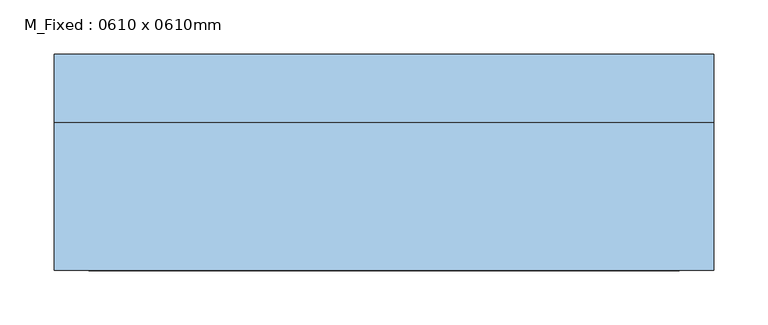
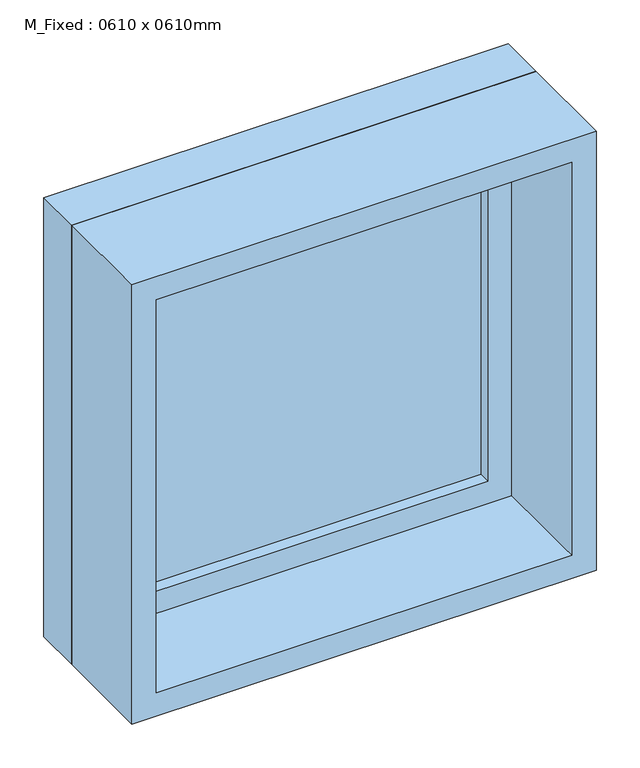
"""IFC4 building model written with IfcOpenShell, lengths in millimetres: window geometry, M_Fixed : 0610 x 0610mm."""

from ifc_helpers import new_model, si_unit, frame, origin, place, context, project, spatial, polyline, outline, extrude, source, transform, mapped, element, save


def m_fixed_0610_x_0610mm_cacddef9(model_context):
    return source(origin(), model_context, "Body", "SweptSolid", [
        extrude(outline(polyline([(-242.0, 78.0), (242.0, 78.0), (242.0, 66.0), (-242.0, 66.0), (-242.0, 78.0)])), frame((0.0, 0.0, 978.0), z_axis=(0.0, 0.0, 1.0), x_axis=(1.0, 0.0, 0.0)), (0.0, 0.0, 1.0), 484.0),
        extrude(outline(polyline([(1506.0, -286.0), (934.0, -286.0), (934.0, 286.0), (1506.0, 286.0), (1506.0, -286.0)]), holes=[polyline([(1462.0, -242.0), (1462.0, 242.0), (978.0, 242.0), (978.0, -242.0), (1462.0, -242.0)])]), frame((0.0, 50.0, 0.0), z_axis=(0.0, 1.0, 0.0), x_axis=(0.0, 0.0, 1.0)), (0.0, 0.0, 1.0), 44.0),
        extrude(outline(polyline([(1525.0, -305.0), (915.0, -305.0), (915.0, 305.0), (1525.0, 305.0), (1525.0, -305.0)]), holes=[polyline([(1506.0, -286.0), (1506.0, 286.0), (934.0, 286.0), (934.0, -286.0), (1506.0, -286.0)])]), frame((0.0, 50.0, 0.0), z_axis=(0.0, 1.0, 0.0), x_axis=(0.0, 0.0, 1.0)), (0.0, 0.0, 1.0), 63.0),
        extrude(outline(polyline([(1525.0, -305.0), (915.0, -305.0), (915.0, 305.0), (1525.0, 305.0), (1525.0, -305.0)]), holes=[polyline([(1493.0, -273.0), (1493.0, 273.0), (947.0, 273.0), (947.0, -273.0), (1493.0, -273.0)])]), frame((0.0, -87.0, 0.0), z_axis=(0.0, 1.0, 0.0), x_axis=(0.0, 0.0, 1.0)), (0.0, 0.0, 1.0), 137.0),
    ])


if __name__ == "__main__":
    model = new_model("IFC4")
    model_context = context("Model", 3, world=origin())
    ifc_project = project(units=[si_unit("LENGTHUNIT", "METRE", prefix="MILLI")], contexts=[model_context])
    site = spatial("IfcSite", under=ifc_project)
    building = spatial("IfcBuilding", under=site)
    placement = place(None, origin())
    m_fixed_0610_x_0610mm_shape = m_fixed_0610_x_0610mm_cacddef9(model_context)
    element("IfcWindow", 1, ObjectType="M_Fixed : 0610 x 0610mm", at=placement, inside=building, context=model_context, shape_type="MappedRepresentation", body=[
        mapped(m_fixed_0610_x_0610mm_shape, transform((0.0, 0.0, 0.0), x_axis=(1.0, 0.0, 0.0), y_axis=(0.0, 1.0, 0.0), z_axis=(0.0, 0.0, 1.0))),
    ])
    save(model, "model.ifc")

# Revit data of these elements
# Type "M_Fixed : 0610 x 0610mm"
#   Type Mark = "12"
#   Height = 610 mm
#   Default Sill Height = 915 mm
#   Width = 610 mm
#   Window Inset = 19 mm
#   Frame Exterior Material = Sash
#   Frame Interior Material = Sash
#   Glass Pane Material = Glass
#   Sash = Sash
#   Wall Closure = (empty or 0)
# Element 1 (IfcWindow, "M_Fixed : 0610 x 0610mm")
#   Materials on its faces: "Sash", "Glass"
# Materials
#   "Sash": class "Wood", colour RGB 136 99 55, transparency 0
#   "Glass": class "Glass", colour RGB 218 227 224, transparency 0.85, Description = "Soda Lime Glass", Cost = 0
